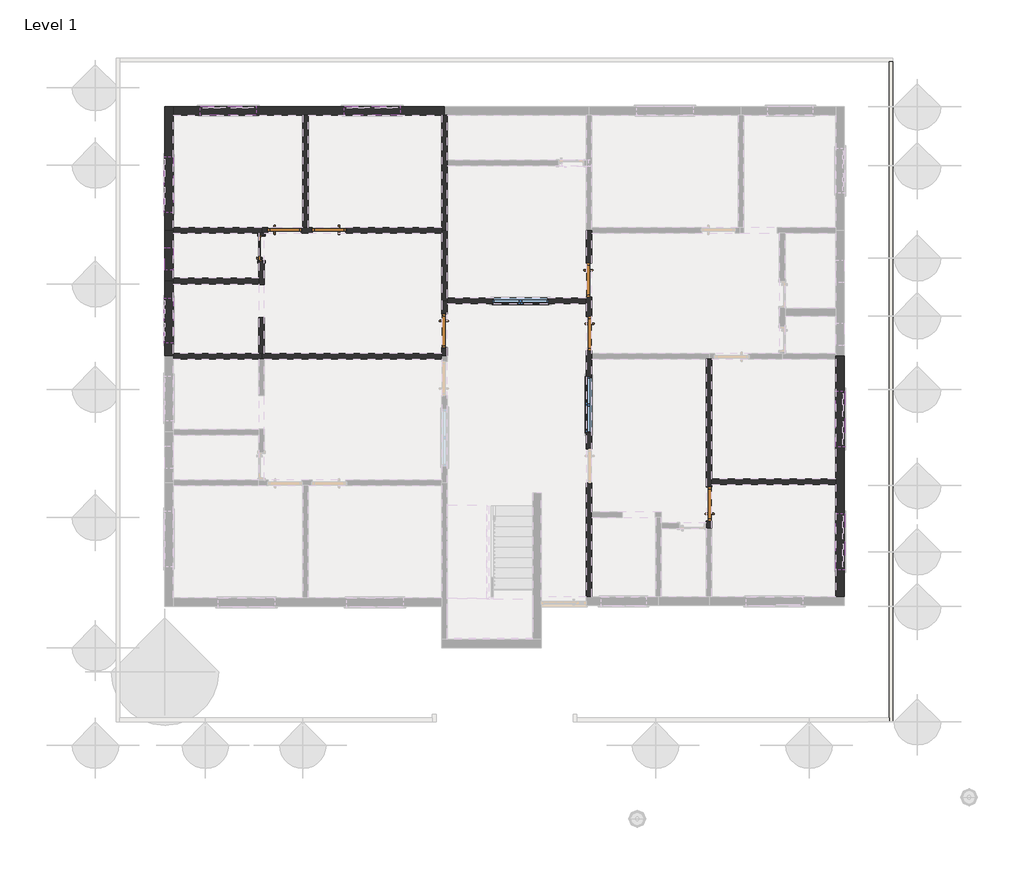
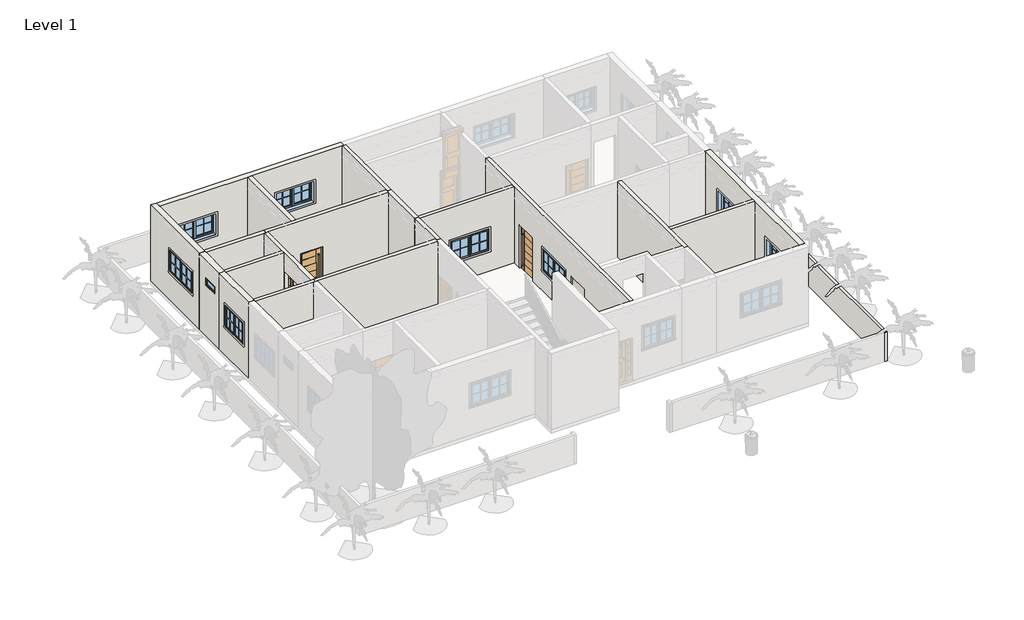
# One storey, part 2 of 5: 20 walls, 9 windows, 7 doors.
# Revit data of these elements (continued)
# Materials (continued)
#   "Aluminum": class "Metal", colour RGB 247 247 247, transparency 0, Description = "Aluminum 6061", Cost = 0
#   "Glass": class "Glass", colour RGB 0 128 192, transparency 0.75, Description = "Soda Lime Glass", Cost = 0
#   "Sash": class "Wood", colour RGB 224 178 126, transparency 0, Cost = 0
#   "Wood - Stained": class "Wood", colour RGB 224 178 126, transparency 0, Cost = 0
#   "Clad - White": class "Wood", colour RGB 242 242 238, transparency 0, Cost = 0
#   "Default Wall": colour RGB 128 128 128, transparency 0, Cost = 0
#   "BRW2": class "Generic", colour RGB 120 120 120, transparency 0, Cost = 0
#   "BW1": class "Generic", colour RGB 120 120 120, transparency 0, Cost = 0
#   "BRW1": class "Generic", colour RGB 120 120 120, transparency 0, Cost = 0
#   "KW2": class "Generic", colour RGB 120 120 120, transparency 0, Cost = 0
#   "KW1": class "Generic", colour RGB 120 120 120, transparency 0, Cost = 0
#   "LVW1": class "Generic", colour RGB 120 120 120, transparency 0, Cost = 0
#   "LVW2": class "Generic", colour RGB 120 120 120, transparency 0, Cost = 0
#   "BRW4": class "Generic", colour RGB 120 120 120, transparency 0, Cost = 0
#   "BRW3": class "Generic", colour RGB 120 120 120, transparency 0, Cost = 0
#   "OW1": class "Generic", colour RGB 120 120 120, transparency 0, Cost = 0
